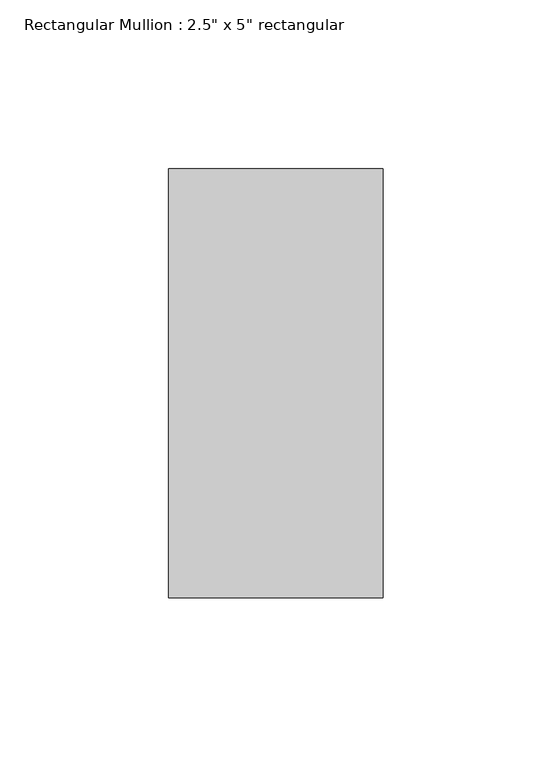
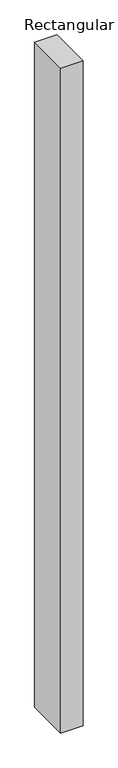
"""IFC4 building model written with IfcOpenShell, lengths in millimetres: member geometry."""

from ifc_helpers import new_model, si_unit, frame, origin, place, context, project, spatial, polyline, outline, extrude, source, transform, mapped, element, save


def member_99d3517c(model_context):
    return source(origin(), model_context, "Body", "SweptSolid", [
        extrude(outline(polyline([(31.75, 63.5), (31.75, -63.5), (-31.75, -63.5), (-31.75, 63.5), (31.75, 63.5)])), frame((0.0, 0.0, -1988.699716), z_axis=(0.0, 0.0, 1.0), x_axis=(1.0, 0.0, 0.0)), (0.0, 0.0, 1.0), 1988.699716),
    ])


if __name__ == "__main__":
    model = new_model("IFC4")
    model_context = context("Model", 3, world=origin())
    ifc_project = project(units=[si_unit("LENGTHUNIT", "METRE", prefix="MILLI")], contexts=[model_context])
    site = spatial("IfcSite", under=ifc_project)
    building = spatial("IfcBuilding", under=site)
    placement = place(None, origin())
    member_shape = member_99d3517c(model_context)
    element("IfcMember", 1, ObjectType="Rectangular Mullion : 2.5\" x 5\" rectangular", at=placement, inside=building, context=model_context, shape_type="MappedRepresentation", body=[
        mapped(member_shape, transform((0.0, 0.0, 0.0), x_axis=(1.0, 0.0, 0.0), y_axis=(0.0, 1.0, 0.0), z_axis=(0.0, 0.0, 1.0))),
    ])
    save(model, "model.ifc")

# Revit data of these elements
# Type "Rectangular Mullion : 2.5\" x 5\" rectangular"
#   built-in parameter 1007304 = 0.416667 (stored number, unit not read)
#   built-in parameter 1007301 = 0.104167 (stored number, unit not read)
#   built-in parameter 1007300 = 0.104167 (stored number, unit not read)
# Element 1 (IfcMember, "Rectangular Mullion : 2.5\" x 5\" rectangular")
#   Materials on its faces: "Aluminum"
# Materials
#   "Aluminum": class "Metal", colour RGB 247 247 247, transparency 0, Description = "Aluminum 6061", Cost = 0
